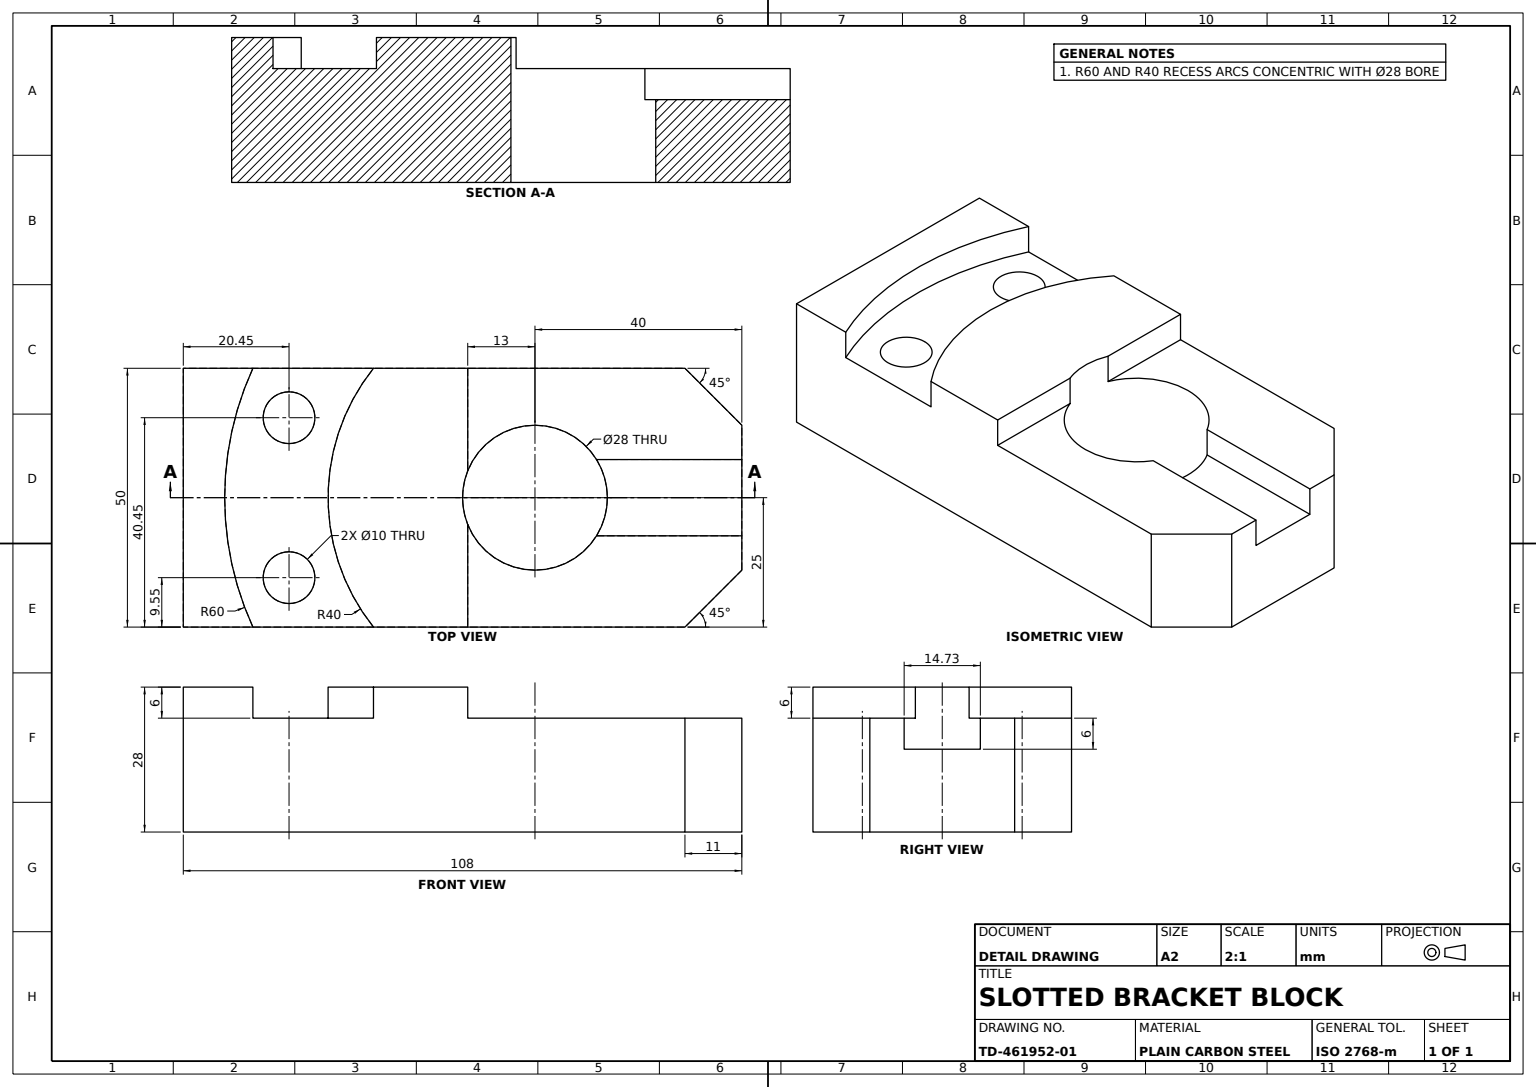
SolidWorks part; units mm, degrees
material "Plain Carbon Steel"
ref_plane "Front Plane" through (0, 0, 0) normal (0, 0, 1) x (1, 0, 0)
ref_plane "Top Plane" through (0, 0, 0) normal (0, 1, 0) x (1, 0, 0)
ref_plane "Right Plane" through (0, 0, 0) normal (1, 0, 0) x (0, 0, -1)
sketch "Base Block Sketch" plane through (0, 0, 0) normal (0, 1, 0) x (1, 0, 0)
  line L1 (-54, 25) -> (54, 25)
  line L2 (-54, 25) -> (-54, -25)
  line L3 (-54, -25) -> (54, -25)
  line L4 (54, 25) -> (54, -25)
  line L5 (-54, 25) -> (54, -25) construction
  line L6 (-54, -25) -> (54, 25) construction
  point P0 (0, 0)
  dimension "D1" = 108
  dimension "D2" = 50
extrude "Base Block 108x50x28" add sketch "Base Block Sketch" along normal mid plane 28
chamfer "End Chamfer 11x45deg" distance 11 angle 45 2 edges at (54, 0, 25) (54, 0, -25)
sketch "Through Bore Sketch" plane through (0, 14, 0) normal (0, 1, 0) x (1, 0, 0)
  line L0 (54, -14) -> (54, 14) construction
  line L1 (43, 25) -> (-54, 25) construction
  circle A0 centre (14, 0) radius 14
  dimension "D1" = 28
  dimension "D2" = 40
  dimension "D3" = 25
extrude "Through Bore" cut sketch "Through Bore Sketch" against normal up to surface (28 mm away) up to face at (14.3333, -14, 0)
sketch "Slot Recess Sketch" plane through (0, 14, 0) normal (0, 1, 0) x (1, 0, 0)
  line L0 (1, 25) -> (1, -25)
  line L1 (43, 25) -> (-54, 25) construction
  line L2 (-54, -25) -> (43, -25) construction
  line L3 (14, 14) -> (14, -14) construction
  line L6 (1, 25) -> (43, 25)
  line L7 (43, 25) -> (54, 14)
  line L8 (54, 14) -> (54, -14)
  line L9 (54, -14) -> (43, -25)
  line L10 (43, -25) -> (1, -25)
  circle A0 centre (14, 0) radius 14 construction
  dimension "D1" = 13
extrude "Slot Recess 6 Deep" cut sketch "Slot Recess Sketch" against normal blind 6
sketch "Arc Recess Sketch" plane through (0, 14, 0) normal (0, 1, 0) x (1, 0, 0)
  line L0 (-54, -25) -> (1, -25) construction
  line L1 (1, 25) -> (-54, 25) construction
  line L2 (-40.5436, -25) -> (-17.225, -25)
  line L3 (-17.225, 25) -> (-40.5436, 25)
  arc A0 (-17.225, 25) -> (-17.225, -25) centre (14, 0) ccw
  arc A1 (-40.5436, 25) -> (-40.5436, -25) centre (14, 0) ccw
  dimension "D1" = 120
  dimension "D2" = 80
extrude "Arc Recess 6 Deep" cut sketch "Arc Recess Sketch" against normal blind 6
sketch "Arc Holes Sketch" plane through (0, 8, 0) normal (0, 1, 0) x (1, 0, 0)
  line L0 (14, 0) -> (-33.5528, 15.4508) construction
  line L1 (14, 0) -> (-33.5528, -15.4508) construction
  line L2 (-53.2503, 0) -> (81.2503, 0) construction
  circle A0 centre (14, 0) radius 50 construction
  circle A1 centre (-33.5528, 15.4508) radius 5
  circle A2 centre (-33.5528, -15.4508) radius 5
  point P9 (14, 0)
  dimension "D1" = 100
  dimension "D4" = 10
  dimension "D5" = 10
  dimension "D2" = 18
  dimension "D3" = 18
extrude "Holes 2xD10 on R100" cut sketch "Arc Holes Sketch" against normal up to surface (22 mm away) up to face at (14, -14, 14)
sketch "Groove Sketch" plane through (0, 8, 0) normal (0, 1, 0) x (1, 0, 0)
  line L0 (25.9047, 7.3673) -> (54, 7.3673)
  line L1 (54, -14) -> (54, 14) construction
  line L2 (25.9047, -7.3673) -> (54, -7.3673)
  line L3 (54, 7.3673) -> (54, -7.3673)
  line L4 (1, -5.1962) -> (1, -25) construction
  arc A0 (1, -5.1962) -> (1, 5.1962) centre (14, 0) ccw construction
  arc A1 (25.9047, -7.3673) -> (25.9047, 7.3673) centre (14, 0) ccw
  dimension "D1" = 24.9047
extrude "Groove 6 Deep" cut sketch "Groove Sketch" against normal blind 6
